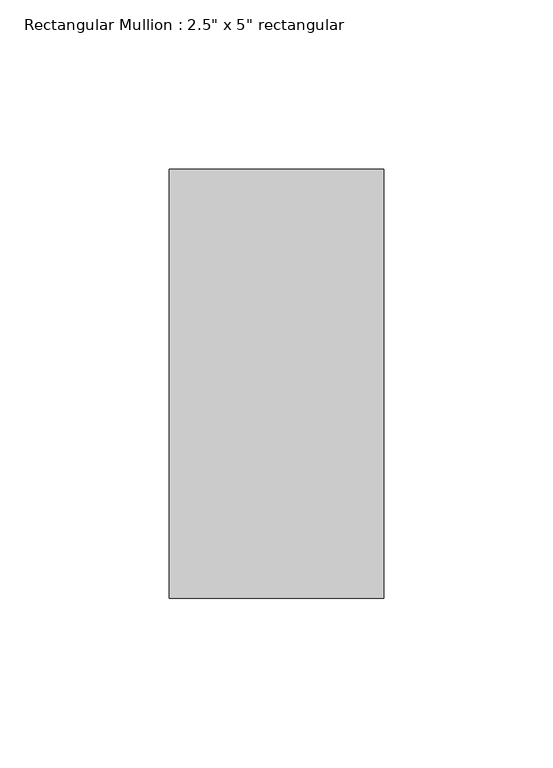
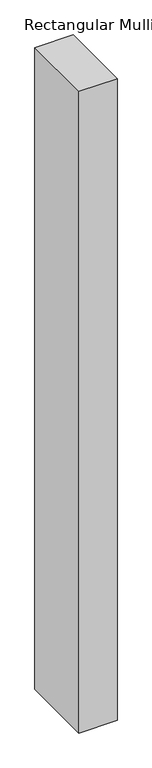
"""IFC4 building model written with IfcOpenShell, lengths in millimetres: member geometry."""

from ifc_helpers import new_model, si_unit, frame, origin, place, context, project, spatial, polyline, outline, extrude, source, transform, mapped, element, save


def member_3285b992(model_context):
    return source(origin(), model_context, "Body", "SweptSolid", [
        extrude(outline(polyline([(0.0, 63.5), (0.0, -63.5), (-63.5, -63.5), (-63.5, 63.5), (0.0, 63.5)])), frame((0.0, 0.0, -1130.3000001), z_axis=(0.0, 0.0, 1.0), x_axis=(1.0, 0.0, 0.0)), (0.0, 0.0, 1.0), 1130.3000001),
    ])


if __name__ == "__main__":
    model = new_model("IFC4")
    model_context = context("Model", 3, world=origin())
    ifc_project = project(units=[si_unit("LENGTHUNIT", "METRE", prefix="MILLI")], contexts=[model_context])
    site = spatial("IfcSite", under=ifc_project)
    building = spatial("IfcBuilding", under=site)
    placement = place(None, origin())
    member_shape = member_3285b992(model_context)
    element("IfcMember", 1, ObjectType="Rectangular Mullion : 2.5\" x 5\" rectangular", at=placement, inside=building, context=model_context, shape_type="MappedRepresentation", body=[
        mapped(member_shape, transform((0.0, 0.0, 0.0), x_axis=(1.0, 0.0, 0.0), y_axis=(0.0, 1.0, 0.0), z_axis=(0.0, 0.0, 1.0))),
    ])
    save(model, "model.ifc")

# Revit data of these elements
# Type "Rectangular Mullion : 2.5\" x 5\" rectangular"
#   built-in parameter 1007304 = 0.416667 (stored number, unit not read)
#   built-in parameter 1007301 = 0.104167 (stored number, unit not read)
#   built-in parameter 1007300 = 0.104167 (stored number, unit not read)
# Element 1 (IfcMember, "Rectangular Mullion : 2.5\" x 5\" rectangular")
#   Materials on its faces: "BLACK COLOUR"
# Materials
#   "BLACK COLOUR": class "Generic", colour RGB 120 120 120, transparency 0, Cost = 0
